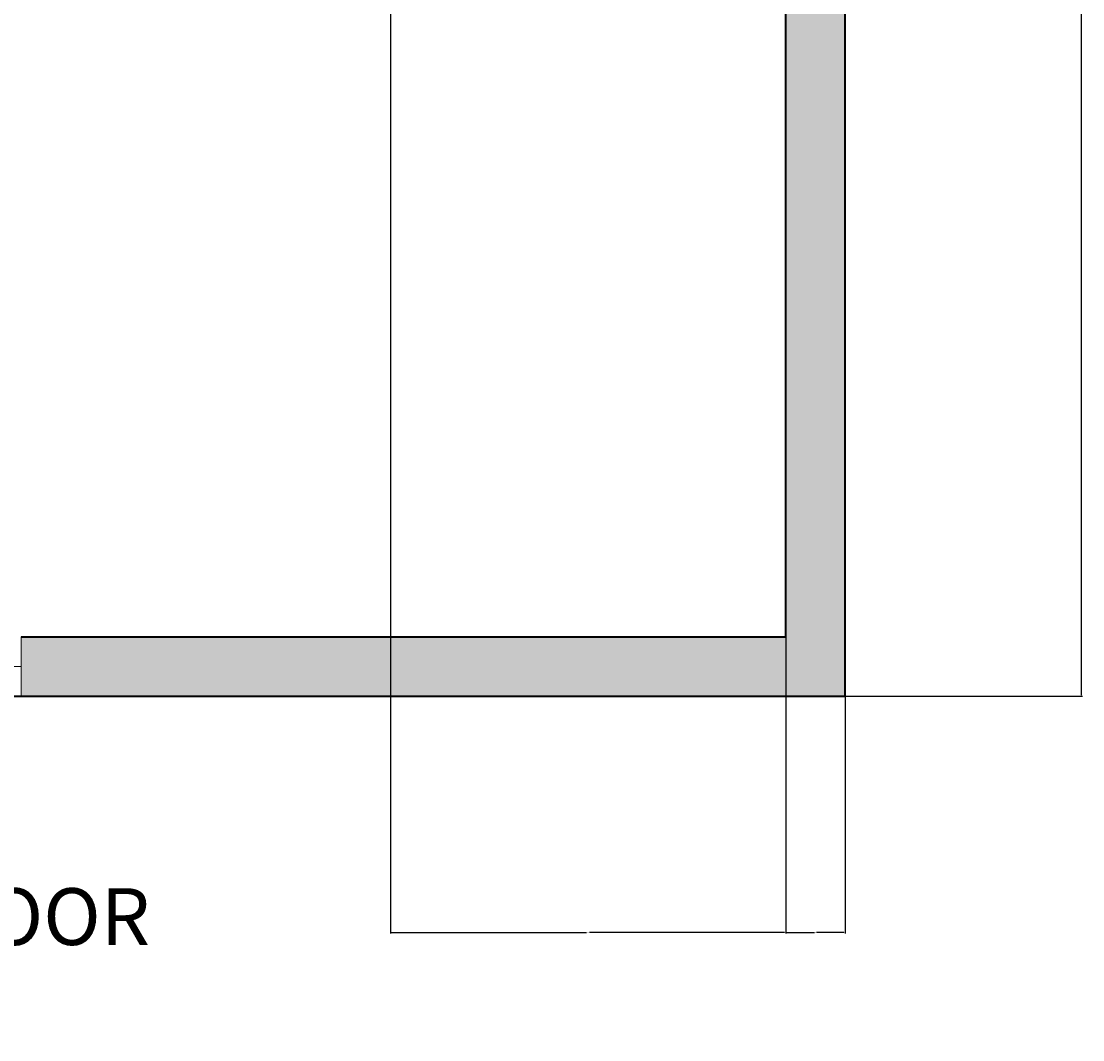
# Model space of a CAD drawing. Units: inches. Extents: x 1568 to 2529, y 2149 to 2897.
# Tile 2 of 16: x 1849 to 2010, y 2149 to 2304. Entities that reach past the tile are written whole.
import ezdxf

# ---------------------------------------------------------------- set-up
doc = ezdxf.new("R2010")
doc.units = ezdxf.units.IN
for name, color, linetype, lineweight in [('A-ANNO-DIMS', 2, 'Continuous', 18), ('A-DOOR', 4, 'Continuous', 18), ('A-WALL-PATT', 172, 'Continuous', 13), ('text', 210, 'Continuous', 18), ('wall', 7, 'Continuous', 35)]:
    doc.layers.add(name, color=color, linetype=linetype, lineweight=lineweight)
doc.styles.get("Standard").update_dxf_attribs({"font": 'arial.ttf'})
doc.dimstyles.get("Standard").update_dxf_attribs({"dimtxt": 0.18, "dimasz": 0.18, "dimexe": 0.18, "dimexo": 0.0625, "dimgap": 0.09, "dimtad": 0, "dimtih": 1, "dimtoh": 1, "dimdec": 4, "dimzin": 0, "dimdsep": 46, "dimtxsty": 'Standard', "dimcen": 0.09, "dimadec": 0, "dimazin": 0, "dimtfac": 1, "dimtdec": 4, "dimtofl": 0, "dimtmove": 0, "dimatfit": 3, "dimfxl": 1, "dimtolj": 1, "dimtzin": 0, "dimarcsym": 0})

# ---------------------------------------------------------------- blocks, each defined once
blk = doc.blocks.new('*D28')
at = {"layer": 'A-ANNO-DIMS', "color": 0, "lineweight": -2, "transparency": 16777216}
for p, q in [((1973.64, 2801.53), (2009.61, 2801.53)), ((2009.43, 2801.35), (2009.43, 2501.71)), ((2009.43, 2201.71), (2009.43, 2501.35)), ((1973.61, 2201.53), (2009.61, 2201.53))]:
    blk.add_line(p, q, dxfattribs=at)
at = {"layer": 'A-ANNO-DIMS', "color": 0, "transparency": 16777216}
for points in [[(2009.4, 2801.35), (2009.46, 2801.35), (2009.43, 2801.53)], [(2009.4, 2201.71), (2009.46, 2201.71), (2009.43, 2201.53)]]:
    blk.add_solid(points, dxfattribs=at)
at = {"layer": 'Defpoints', "color": 0, "transparency": 16777216}
for p in [(1973.58, 2801.53), (2009.43, 2801.53), (1973.55, 2201.53)]:
    blk.add_point(p, dxfattribs=at)
at = {"layer": 'A-ANNO-DIMS', "color": 0, "transparency": 16777216, "insert": (2009.43, 2501.53), "char_height": 0.18, "attachment_point": 5}
blk.add_mtext('\\A1;600', dxfattribs=at)
blk = doc.blocks.new('*D32')
at = {"layer": 'A-ANNO-DIMS', "color": 0, "lineweight": -2, "transparency": 16777216}
for p, q in [((1964.55, 2792.47), (1964.55, 2165.5)), ((1904.55, 2753.4), (1904.55, 2165.5)), ((1904.73, 2165.68), (1934.33, 2165.68)), ((1964.37, 2165.68), (1934.77, 2165.68))]:
    blk.add_line(p, q, dxfattribs=at)
at = {"layer": 'A-ANNO-DIMS', "color": 0, "transparency": 16777216}
for points in [[(1904.73, 2165.71), (1904.73, 2165.65), (1904.55, 2165.68)], [(1964.37, 2165.71), (1964.37, 2165.65), (1964.55, 2165.68)]]:
    blk.add_solid(points, dxfattribs=at)
at = {"layer": 'Defpoints', "color": 0, "transparency": 16777216}
for p in [(1964.55, 2792.53), (1904.55, 2753.46), (1964.55, 2165.68)]:
    blk.add_point(p, dxfattribs=at)
at = {"layer": 'A-ANNO-DIMS', "color": 0, "transparency": 16777216, "insert": (1934.55, 2165.68), "char_height": 0.18, "attachment_point": 5}
blk.add_mtext('\\A1;60', dxfattribs=at)
blk = doc.blocks.new('*D46')
at = {"layer": 'A-ANNO-DIMS', "color": 0, "lineweight": -2, "transparency": 16777216}
for p, q in [((1964.55, 2210.47), (1964.55, 2165.5)), ((1973.55, 2201.47), (1973.55, 2165.5)), ((1964.73, 2165.68), (1968.9, 2165.68)), ((1973.37, 2165.68), (1969.2, 2165.68))]:
    blk.add_line(p, q, dxfattribs=at)
at = {"layer": 'A-ANNO-DIMS', "color": 0, "transparency": 16777216}
for points in [[(1964.73, 2165.71), (1964.73, 2165.65), (1964.55, 2165.68)], [(1973.37, 2165.71), (1973.37, 2165.65), (1973.55, 2165.68)]]:
    blk.add_solid(points, dxfattribs=at)
at = {"layer": 'Defpoints', "color": 0, "transparency": 16777216}
for p in [(1964.55, 2210.53), (1973.55, 2201.53), (1973.55, 2165.68)]:
    blk.add_point(p, dxfattribs=at)
at = {"layer": 'A-ANNO-DIMS', "color": 0, "transparency": 16777216, "insert": (1969.05, 2165.68), "char_height": 0.18, "attachment_point": 5}
blk.add_mtext('\\A1;9', dxfattribs=at)

msp = doc.modelspace()

# ---------------------------------------------------------------- hatches: boundary and pattern name
at = {"layer": 'A-WALL-PATT'}
h = msp.add_hatch(color=256, dxfattribs=at)
h.dxf.hatch_style = 1
h.paths.add_polyline_path([(1973.5509, 2330.532), (1964.5509, 2330.532), (1964.5509, 2210.532), (1848.5145, 2210.532), (1848.5145, 2201.532), (1973.5509, 2201.532)])
h.paths.add_polyline_path([(1622.5509, 2330.532), (1613.5509, 2330.532), (1613.5509, 2201.532), (1752.5179, 2201.532), (1752.5179, 2210.532), (1622.5509, 2210.532)])

# ---------------------------------------------------------------- linework, layer by layer
at = {"layer": 'A-DOOR'}
for p, q in [((1848.5145, 2210.532), (1848.5145, 2201.532)), ((1752.5179, 2206.032), (1848.5145, 2206.032))]:
    msp.add_line(p, q, dxfattribs=at)
at = {"layer": 'wall'}
msp.add_lwpolyline([(1613.5509, 2201.532), (1973.5509, 2201.532), (1973.5509, 2801.532), (1613.5509, 2801.532)], close=True, dxfattribs=at)
msp.add_lwpolyline([(1848.5145, 2210.532), (1964.5509, 2210.532), (1964.5509, 2330.532)], dxfattribs=at)

# ---------------------------------------------------------------- texts
at = {"layer": 'text', "insert": (1778.1838, 2172.397), "char_height": 8.628146, "attachment_point": 1}
msp.add_mtext_dynamic_manual_height_columns('GROUND FLOOR PLAN', width=94.297369, gutter_width=43.1407, heights=[0], dxfattribs=at)

# ---------------------------------------------------------------- dimensions: what is measured, and where the dimension line sits
at = {"layer": 'A-ANNO-DIMS'}
dim = msp.add_linear_dim(base=(2009.4302, 2801.532), p1=(1973.5509, 2201.532), p2=(1973.5802, 2801.532), angle=90, dimstyle='Standard', override={"dimdec": 0, "dimlfac": 1, "dimrnd": 0, "dimzin": 0, "dimdsep": 46, "dimlunit": 2}, dxfattribs=at)
dim.commit()
dim.dimension.update_dxf_attribs({"geometry": '*D28', "text_midpoint": (2009.4302, 2501.532)})
for base, p1, p2, picture, middle in [((1964.5509, 2165.682), (1904.5509, 2753.4635), (1964.5509, 2792.532), '*D32', (1934.5509, 2165.682)), ((1973.5509, 2165.682), (1964.5509, 2210.532), (1973.5509, 2201.532), '*D46', (1969.0509, 2165.682))]:
    dim = msp.add_linear_dim(base=base, p1=p1, p2=p2, dimstyle='Standard', override={"dimdec": 0, "dimlfac": 1, "dimrnd": 0, "dimzin": 0, "dimdsep": 46, "dimlunit": 2}, dxfattribs=at)
    dim.commit()
    dim.dimension.update_dxf_attribs({"geometry": picture, "text_midpoint": middle})

doc.saveas('drawing.dxf')
